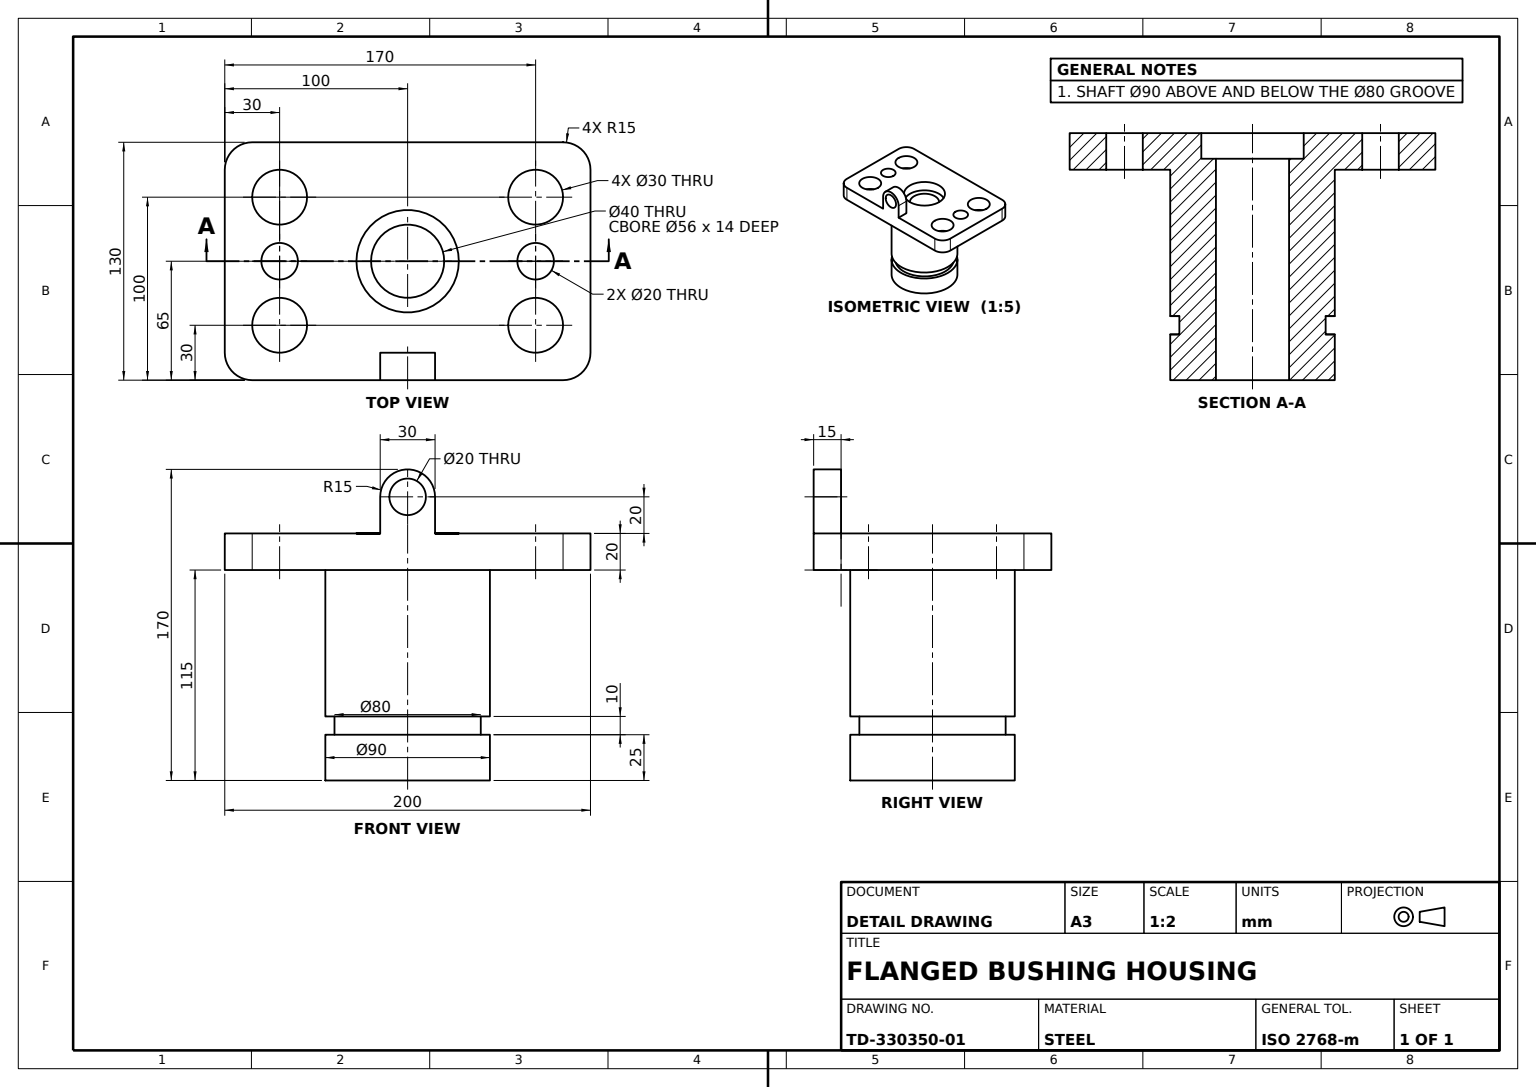
from build123d import *

# Parameters (mm, degrees)
MOUNTING_PLATE_SKETCH_R         = 15
MOUNTING_PLATE_SKETCH_R_2       = 10
MOUNTING_PLATE_SKETCH_R_3       = 45
MOUNTING_PLATE_SKETCH_R_4       = 28
MOUNTING_PLATE_200X130X20_DEPTH = 20
PIVOT_LUG_SKETCH_R              = 10
PIVOT_LUG_DEPTH                 = 15
RING_BOSS_SKETCH_R              = 28
RING_BOSS_SKETCH_R_2            = 20
RING_BOSS_6MM_DEPTH             = 6


with BuildPart() as part:
    # Shaft Profile Sketch → Grooved Shaft Revolve (revolve)
    with BuildSketch(Plane.XY):
        Polygon((-45, 57.5), (-45, -22.5), (-40, -22.5), (-40, -32.5), (-45, -32.5), (-45, -57.5), (-20, -57.5), (-20, 57.5), align=None)
    revolve(axis=Axis((0, 146.177983413, 0), (0, -1, 0)))

    # Mounting Plate Sketch → Mounting Plate 200x130x20 (add)
    # profile 1 of 2: a face of its own
    with BuildSketch(Plane(origin=(0, 57.5, 0), x_dir=(1, 0, 0), z_dir=(0, 1, 0))):
        with BuildLine():
            ThreePointArc((85, 65), (95.606601718, 60.606601718), (100, 50))
            Line((100, 50), (100, -50))
            ThreePointArc((100, -50), (95.606601718, -60.606601718), (85, -65))
            Line((85, -65), (-85, -65))
            ThreePointArc((-85, -65), (-95.606601718, -60.606601718), (-100, -50))
            Line((-100, -50), (-100, 50))
            ThreePointArc((-100, 50), (-95.606601718, 60.606601718), (-85, 65))
            Line((-85, 65), (85, 65))
        make_face()
        with Locations(Location((70, 35, 0), (0, 0, 180))):
            Circle(MOUNTING_PLATE_SKETCH_R, mode=Mode.SUBTRACT)
        with Locations(Location((70, -35, 0), (0, 0, 180))):
            Circle(MOUNTING_PLATE_SKETCH_R, mode=Mode.SUBTRACT)
        with Locations(Location((-70, 0, 0), (0, 0, 180))):
            Circle(MOUNTING_PLATE_SKETCH_R_2, mode=Mode.SUBTRACT)
        with Locations(Location((-70, -35, 0), (0, 0, 180))):
            Circle(MOUNTING_PLATE_SKETCH_R, mode=Mode.SUBTRACT)
        with Locations(Location((-70, 35, 0), (0, 0, 180))):
            Circle(MOUNTING_PLATE_SKETCH_R, mode=Mode.SUBTRACT)
        with Locations(Location((70, 0, 0), (0, 0, 180))):
            Circle(MOUNTING_PLATE_SKETCH_R_2, mode=Mode.SUBTRACT)
        with Locations(Location((0, 0, 0), (0, 0, 180))):
            Circle(MOUNTING_PLATE_SKETCH_R_3, mode=Mode.SUBTRACT)
    # profile 2 of 2: a face of its own
    with BuildSketch(Plane(origin=(0, 57.5, 0), x_dir=(1, 0, 0), z_dir=(0, 1, 0))):
        with Locations(Location((0, 0, 0), (0, 0, 180))):
            Circle(MOUNTING_PLATE_SKETCH_R_3)
        with Locations(Location((0, 0, 0), (0, 0, 180))):
            Circle(MOUNTING_PLATE_SKETCH_R_4, mode=Mode.SUBTRACT)
    extrude(amount=MOUNTING_PLATE_200X130X20_DEPTH)

    # Pivot Lug Sketch → Pivot Lug (add)
    with BuildSketch(Plane.XY.offset(65)):
        with BuildLine():
            Line((15, 97.5), (15, 77.5))
            Line((15, 77.5), (-15, 77.5))
            Line((-15, 77.5), (-15, 97.5))
            ThreePointArc((-15, 97.5), (0, 112.5), (15, 97.5))
        make_face()
        with Locations((0, 97.5)):
            Circle(PIVOT_LUG_SKETCH_R, mode=Mode.SUBTRACT)
    extrude(amount=-PIVOT_LUG_DEPTH)

    # Ring Boss Sketch → Ring Boss 6mm (add)
    with BuildSketch(Plane(origin=(0, 57.5, 0), x_dir=(1, 0, 0), z_dir=(0, 1, 0))):
        with Locations(Location((0, 0, 0), (0, 0, 180))):
            Circle(RING_BOSS_SKETCH_R)
        with Locations(Location((0, 0, 0), (0, 0, 180))):
            Circle(RING_BOSS_SKETCH_R_2, mode=Mode.SUBTRACT)
    extrude(amount=RING_BOSS_6MM_DEPTH)


solid = part.part
